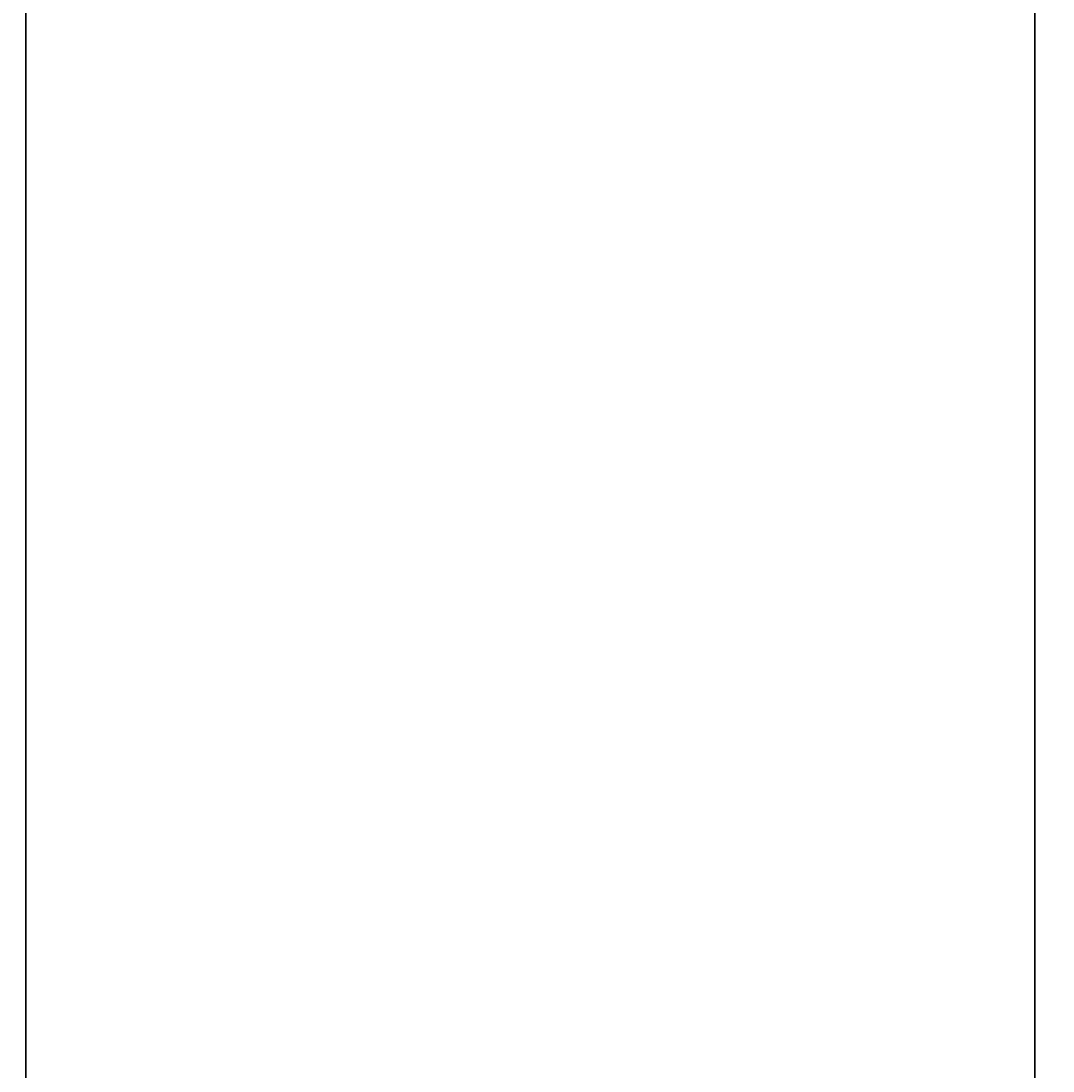
# Model space of a CAD drawing. Units: inches. Extents: x -61 to 1599, y -1316 to 257.
# Tile 15 of 204: x -61 to 16, y -868 to -790. Entities that reach past the tile are written whole.
import ezdxf

# ---------------------------------------------------------------- set-up
doc = ezdxf.new("R2010")
doc.units = ezdxf.units.IN
doc.header["$MEASUREMENT"] = 0
doc.layers.add('A-ANNO-DIMS', color=2, linetype='Continuous', lineweight=18)
doc.layers.add('WALLS', color=4, linetype='Continuous', lineweight=35)
doc.styles.get("Standard").update_dxf_attribs({"font": 'arial.ttf'})
doc.dimstyles.get("Standard").update_dxf_attribs({"dimtxt": 0.18, "dimasz": 0.18, "dimexe": 0.18, "dimexo": 0.0625, "dimgap": 0.09, "dimtad": 0, "dimtih": 1, "dimtoh": 1, "dimdec": 0, "dimzin": 0, "dimdsep": 46, "dimlunit": 3, "dimtxsty": 'Standard', "dimcen": 0.09, "dimadec": 0, "dimazin": 0, "dimtfac": 1, "dimtdec": 0, "dimtofl": 0, "dimtmove": 0, "dimatfit": 3, "dimfxl": 1, "dimtolj": 1, "dimtzin": 0, "dimarcsym": 0})

# ---------------------------------------------------------------- blocks, each defined once
blk = doc.blocks.new('*D687')
at = {"layer": 'A-ANNO-DIMS', "color": 0, "lineweight": -2, "transparency": 16777216}
for p, q in [((289.418, 181.677), (-61.077, 181.677)), ((-60.897, 181.497), (-60.897, -528.952)), ((-60.897, -1239.765), (-60.897, -529.316)), ((319.64, -1239.945), (-61.077, -1239.945))]:
    blk.add_line(p, q, dxfattribs=at)
at = {"layer": 'A-ANNO-DIMS', "color": 0, "transparency": 16777216}
for points in [[(-60.927, 181.497), (-60.867, 181.497), (-60.897, 181.677)], [(-60.927, -1239.765), (-60.867, -1239.765), (-60.897, -1239.945)]]:
    blk.add_solid(points, dxfattribs=at)
at = {"layer": 'DEFPOINTS', "color": 0, "transparency": 16777216}
for p in [(289.481, 181.677), (-60.897, -1239.945), (319.703, -1239.945)]:
    blk.add_point(p, dxfattribs=at)
at = {"layer": 'A-ANNO-DIMS', "color": 0, "transparency": 16777216, "insert": (-60.897, -529.134), "char_height": 0.18, "attachment_point": 5}
blk.add_mtext('\\A1;1421.6', dxfattribs=at)
blk = doc.blocks.new('*D693')
at = {"layer": 'A-ANNO-DIMS', "color": 0, "lineweight": -2, "transparency": 16777216}
for p, q in [((14.64, -616.945), (-61.077, -616.945)), ((-60.897, -617.125), (-60.897, -916.263)), ((-60.897, -1215.765), (-60.897, -916.626)), ((14.64, -1215.945), (-61.077, -1215.945))]:
    blk.add_line(p, q, dxfattribs=at)
at = {"layer": 'A-ANNO-DIMS', "color": 0, "transparency": 16777216}
for points in [[(-60.927, -617.125), (-60.867, -617.125), (-60.897, -616.945)], [(-60.927, -1215.765), (-60.867, -1215.765), (-60.897, -1215.945)]]:
    blk.add_solid(points, dxfattribs=at)
at = {"layer": 'DEFPOINTS', "color": 0, "transparency": 16777216}
for p in [(-60.897, -616.945), (14.703, -616.945), (14.703, -1215.945)]:
    blk.add_point(p, dxfattribs=at)
at = {"layer": 'A-ANNO-DIMS', "color": 0, "transparency": 16777216, "insert": (-60.897, -916.445), "char_height": 0.18, "attachment_point": 5}
blk.add_mtext('\\A1;599', dxfattribs=at)

msp = doc.modelspace()

# ---------------------------------------------------------------- linework, layer by layer
at = {"layer": 'WALLS'}
msp.add_line((14.7028, -616.9446), (14.7028, -1215.9446), dxfattribs=at)

# ---------------------------------------------------------------- dimensions: what is measured, and where the dimension line sits
at = {"layer": 'A-ANNO-DIMS'}
for base, p1, p2, override, picture, middle in [((-60.8972, -1239.9446), (289.4807, 181.6771), (319.7028, -1239.9446), {"dimdec": 1, "dimlfac": 1, "dimrnd": 0, "dimzin": 0, "dimdsep": 46, "dimlunit": 2}, '*D687', (-60.8972, -529.1337)), ((-60.8972, -616.9446), (14.7028, -1215.9446), (14.7028, -616.9446), {"dimdec": 0, "dimlfac": 1, "dimrnd": 0, "dimzin": 0, "dimdsep": 46, "dimlunit": 2}, '*D693', (-60.8972, -916.4446))]:
    dim = msp.add_linear_dim(base=base, p1=p1, p2=p2, angle=90, dimstyle='Standard', override=override, dxfattribs=at)
    dim.commit()
    dim.dimension.update_dxf_attribs({"geometry": picture, "text_midpoint": middle})

doc.saveas('drawing.dxf')
